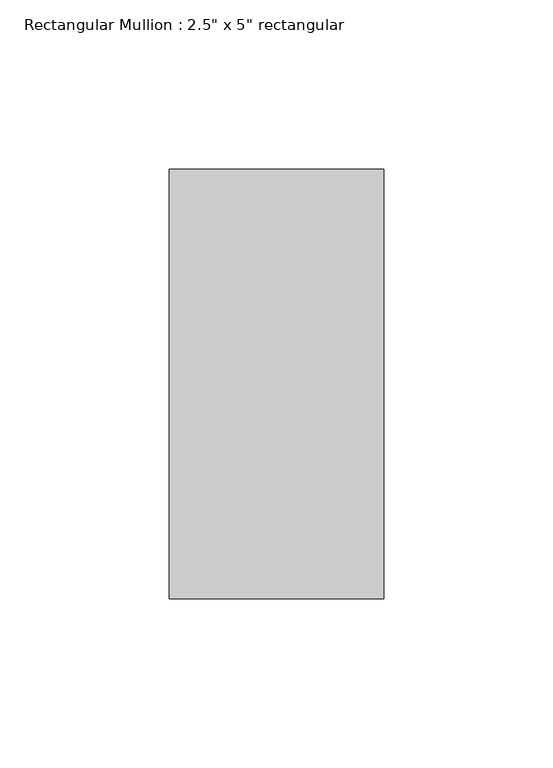
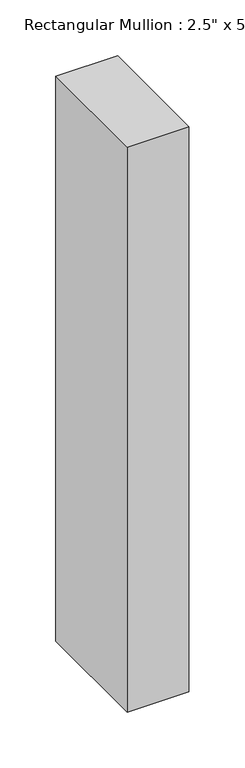
"""IFC4 building model written with IfcOpenShell, lengths in millimetres: member geometry."""

from ifc_helpers import new_model, si_unit, frame, origin, place, context, project, spatial, polyline, outline, extrude, source, transform, mapped, element, save


def member_e58ec603(model_context):
    return source(origin(), model_context, "Body", "SweptSolid", [
        extrude(outline(polyline([(0.0, 63.5), (0.0, -63.5), (-63.5, -63.5), (-63.5, 63.5), (0.0, 63.5)])), frame((0.0, 0.0, -616.070328), z_axis=(0.0, 0.0, 1.0), x_axis=(1.0, 0.0, 0.0)), (0.0, 0.0, 1.0), 616.070328),
    ])


if __name__ == "__main__":
    model = new_model("IFC4")
    model_context = context("Model", 3, world=origin())
    ifc_project = project(units=[si_unit("LENGTHUNIT", "METRE", prefix="MILLI")], contexts=[model_context])
    site = spatial("IfcSite", under=ifc_project)
    building = spatial("IfcBuilding", under=site)
    placement = place(None, origin())
    member_shape = member_e58ec603(model_context)
    element("IfcMember", 1, ObjectType="Rectangular Mullion : 2.5\" x 5\" rectangular", at=placement, inside=building, context=model_context, shape_type="MappedRepresentation", body=[
        mapped(member_shape, transform((0.0, 0.0, 0.0), x_axis=(1.0, 0.0, 0.0), y_axis=(0.0, 1.0, 0.0), z_axis=(0.0, 0.0, 1.0))),
    ])
    save(model, "model.ifc")

# Revit data of these elements
# Type "Rectangular Mullion : 2.5\" x 5\" rectangular"
#   built-in parameter 1007304 = 0.416667 (stored number, unit not read)
#   built-in parameter 1007301 = 0.104167 (stored number, unit not read)
#   built-in parameter 1007300 = 0.104167 (stored number, unit not read)
# Element 1 (IfcMember, "Rectangular Mullion : 2.5\" x 5\" rectangular")
#   Materials on its faces: "Aluminum"
# Materials
#   "Aluminum": class "Metal", colour RGB 247 247 247, transparency 0, Description = "Aluminum 6061", Cost = 0
